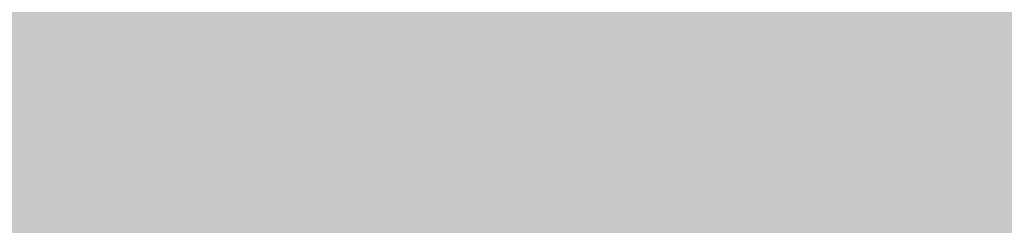
# Model space of a CAD drawing. Units: feet. Extents: x 3168 to 4724, y 827 to 1477.
# Tile 154 of 256: x 3301.19778 to 3301.26573, y 1099.00068 to 1099.01485. Entities that reach past the tile are written whole.
import ezdxf

# ---------------------------------------------------------------- set-up
doc = ezdxf.new("R2010")
doc.units = ezdxf.units.FT
doc.layers.add('A-ELEV', color=7, linetype='Continuous', lineweight=35)
doc.layers.add('A-ELEV-PATT', color=8, linetype='Continuous', lineweight=13)

msp = doc.modelspace()

# ---------------------------------------------------------------- hatches: boundary and pattern name
at = {"layer": 'A-ELEV-PATT'}
h = msp.add_hatch(color=256, dxfattribs=at)
h.dxf.hatch_style = 1
edge = h.paths.add_edge_path()
edge.add_ellipse((3552.905762, 979.220141), major_axis=(36.744924, 0), ratio=0.484848485, start_angle=0, end_angle=360)
edge = h.paths.add_edge_path()
edge.add_ellipse((3559.891637, 929.252282), major_axis=(36.744924, 0), ratio=0.484848485, start_angle=0, end_angle=360)
edge = h.paths.add_edge_path()
edge.add_line((3299.31681, 1198.606081), (3479.916714, 1198.606081))
edge.add_line((3479.916714, 1198.606081), (3479.916714, 1209.86857))
edge.add_spline(control_points=[(3479.916714, 1209.86857), (3464.301157, 1209.86857), (3448.685601, 1209.86857), (3410.949139, 1209.86857), (3388.828234, 1209.86857), (3355.646876, 1209.86857), (3344.586423, 1209.86857), (3327.995745, 1209.86857), (3322.465518, 1209.86857), (3314.170179, 1209.86857), (3311.405066, 1209.86857), (3307.257396, 1209.86857), (3305.874839, 1209.86857), (3303.801005, 1209.86857), (3303.109726, 1209.86857), (3302.072809, 1209.86857), (3301.72717, 1209.86857), (3301.208711, 1209.86857), (3301.035891, 1209.86857), (3300.776662, 1209.86857), (3300.690252, 1209.86857), (3300.560638, 1209.86857), (3300.517433, 1209.86857), (3300.452625, 1209.86857), (3300.431023, 1209.86857), (3300.398619, 1209.86857), (3300.387818, 1209.86857), (3300.366216, 1209.86857), (3300.345676, 1209.86857), (3300.345548, 1209.86857), (3300.345505, 1209.86857), (3300.343304, 1209.86857), (3300.341146, 1209.868571), (3300.337909, 1209.868571), (3300.33683, 1209.868572), (3300.333942, 1209.868573), (3300.332133, 1209.868574), (3300.325515, 1209.868577), (3300.320706, 1209.868581), (3300.310925, 1209.868592), (3300.305952, 1209.868598), (3300.290511, 1209.868623), (3300.280045, 1209.868646), (3300.232425, 1209.868777), (3300.195298, 1209.868954), (3299.951068, 1209.870608), (3299.744824, 1209.874326), (3299.436827, 1209.883257), (3299.334389, 1209.886792), (3299.181079, 1209.89292), (3299.130033, 1209.895099), (3298.652217, 1209.916801), (3298.22946, 1209.945718), (3297.601631, 1210.002367), (3297.393404, 1210.023464), (3297.082652, 1210.058309), (3296.979332, 1210.070458), (3296.292954, 1210.154861), (3295.718148, 1210.243356), (3294.868717, 1210.39885), (3294.5877, 1210.454478), (3294.169341, 1210.543349), (3294.030415, 1210.573878), (3291.707149, 1211.1012), (3289.65359, 1211.813435), (3285.776259, 1213.563988), (3283.95141, 1214.603478), (3280.512159, 1216.98008), (3278.897241, 1218.317592), (3276.379914, 1220.829489), (3275.416042, 1221.917738), (3274.039342, 1223.7077), (3273.581043, 1224.349535), (3273.143228, 1225.016316)], knot_values=[39.119033, 39.119033, 39.119033, 39.119033, 39.286353, 39.286353, 39.523379, 39.523379, 39.641892, 39.641892, 39.701148, 39.701148, 39.730777, 39.730777, 39.745591, 39.745591, 39.752998, 39.752998, 39.756701, 39.756701, 39.758553, 39.758553, 39.759479, 39.759479, 39.759942, 39.759942, 39.760173, 39.760173, 39.760289, 39.760289, 39.760405, 39.760405, 39.760463, 39.760463, 39.763389, 39.763389, 39.764851, 39.764851, 39.767304, 39.767304, 39.773825, 39.773825, 39.78057, 39.78057, 39.79477, 39.79477, 39.845194, 39.845194, 40.126715, 40.126715, 40.267476, 40.267476, 40.337856, 40.337856, 40.927023, 40.927023, 41.221606, 41.221606, 41.368898, 41.368898, 42.202622, 42.202622, 42.619485, 42.619485, 42.827916, 42.827916, 46.118323, 46.118323, 49.408731, 49.408731, 52.699139, 52.699139, 54.927489, 54.927489, 56.104228, 56.104228, 56.104228, 56.104228], weights=[1, 1, 1, 1, 1, 1, 1, 1, 1, 1, 1, 1, 1, 1, 1, 1, 1, 1, 1, 1, 1, 1, 1, 1, 1, 1, 1, 1, 1, 1, 1, 1, 1, 1, 1, 1, 1, 1, 1, 1, 1, 1, 1, 1, 1, 1, 1, 1, 1, 1, 1, 1, 1, 1, 1, 1, 1, 1, 1, 1, 1, 1, 1, 1, 1, 1, 1, 1, 1, 1, 1, 1, 1, 1], degree=3, periodic=0)
edge.add_line((3273.143228, 1225.016316), (3273.143228, 1099.016316))
edge.add_line((3273.143228, 1099.016316), (3299.31681, 1099.016316))
edge.add_line((3299.31681, 1099.016316), (3299.31681, 1198.606081))
edge = h.paths.add_edge_path()
edge.add_line((3304.758443, 1324.15806), (3479.916714, 1324.15806))
edge.add_line((3479.916714, 1324.15806), (3479.916714, 1335.714618))
edge.add_line((3479.916714, 1335.714618), (3269.161628, 1335.714618))
edge.add_spline(control_points=[(3269.161628, 1335.714618), (3264.024231, 1335.714618), (3258.364118, 1328.958189), (3259.264311, 1323.900274)], knot_values=[0, 0, 0, 0, 15.412191, 15.412191, 15.412191, 15.412191], degree=3, periodic=0)
edge.add_line((3259.264311, 1323.900274), (3265.516849, 1288.769135))
edge.add_line((3265.516849, 1288.769135), (3275.265103, 1261.545626))
edge.add_line((3275.265103, 1261.545626), (3304.758443, 1261.545626))
edge.add_line((3304.758443, 1261.545626), (3304.758443, 1324.15806))
h = msp.add_hatch(color=256, dxfattribs=at)
h.dxf.hatch_style = 1
h.paths.add_polyline_path([(3384.525247, 1099.016316), (3335.029168, 1099.016316), (3299.31681, 1099.016316), (3273.143228, 1099.016316), (3217.565364, 1099.016316), (3168.069285, 827.11626), (3335.029168, 827.11626)])

# ---------------------------------------------------------------- linework, layer by layer
at = {"layer": 'A-ELEV'}
msp.add_open_spline([(3808.5202, 1099.016316), (3808.5202, 1141.413235), (3808.5202, 1183.810154), (3808.5202, 1226.635324), (3808.5202, 1227.063576), (3808.5202, 1227.491828), (3811.491871, 1248.994673), (3814.463542, 1270.497518), (3817.46523, 1292.217564), (3817.495247, 1292.434764), (3817.525264, 1292.651964), (3817.572801, 1310.106748), (3817.620339, 1327.561532), (3817.667877, 1345.016316), (3817.667877, 1345.457962), (3817.667877, 1345.899608), (3817.667877, 1346.456047), (3817.667877, 1346.57084), (3817.667877, 1346.752887), (3817.667877, 1346.820142), (3817.667877, 1346.93487), (3817.667877, 1346.982345), (3817.667877, 1347.038587), (3817.667877, 1347.047356), (3817.667877, 1347.073661), (3817.667877, 1347.059303), (3817.667877, 1347.061545), (3817.667876, 1347.062667), (3817.667875, 1347.066031), (3817.667874, 1347.068274), (3817.66787, 1347.075001), (3817.667866, 1347.079486), (3817.667849, 1347.092937), (3817.667833, 1347.101902), (3817.667766, 1347.12879), (3817.667699, 1347.146705), (3817.667432, 1347.200421), (3817.667165, 1347.236192), (3817.6661, 1347.343385), (3817.665038, 1347.414686), (3817.660812, 1347.628095), (3817.656608, 1347.769708), (3817.63997, 1348.192487), (3817.623509, 1348.471586), (3817.559094, 1349.300067), (3817.496121, 1349.840588), (3817.255432, 1351.424156), (3817.026318, 1352.428785), (3816.306871, 1354.888914), (3815.743745, 1356.268727), (3814.463959, 1358.81921), (3813.746413, 1359.990968), (3812.195838, 1362.172343), (3811.362245, 1363.182124), (3809.588836, 1365.069009), (3808.648816, 1365.946105), (3806.654262, 1367.579616), (3805.599702, 1368.336154), (3803.352891, 1369.722327), (3802.160535, 1370.352386), (3799.600813, 1371.453586), (3798.232688, 1371.925481), (3795.280084, 1372.634624), (3793.693148, 1372.872068), (3791.869441, 1372.92648), (3791.740861, 1372.92922), (3791.353371, 1372.934101), (3791.092707, 1372.932901), (3790.304116, 1372.915068), (3789.769543, 1372.884195), (3789.20919, 1372.830236), (3789.190622, 1372.828424), (3789.134892, 1372.822912), (3789.097705, 1372.819137), (3789.048445, 1372.814008), (3789.0364, 1372.812743), (3789.000256, 1372.808918), (3788.976147, 1372.806325), (3788.949405, 1372.803404), (3788.946786, 1372.803118), (3788.942567, 1372.802655), (3788.940967, 1372.80248), (3788.938572, 1372.802217), (3788.937777, 1372.802129), (3788.935391, 1372.801867), (3788.867535, 1372.794402), (3788.756866, 1372.782228), (3788.701532, 1372.776141), (3788.53553, 1372.75788), (3788.424861, 1372.745707), (3788.092856, 1372.709185), (3787.871519, 1372.684837), (3787.207509, 1372.611793), (3786.764835, 1372.563097), (3785.436814, 1372.417009), (3784.551467, 1372.319617), (3781.895425, 1372.027442), (3780.12473, 1371.832658), (3774.812646, 1371.248307), (3771.271256, 1370.858739), (3760.647088, 1369.690037), (3753.56431, 1368.910902), (3732.315973, 1366.573498), (3718.150416, 1365.015228), (3694.006758, 1362.359326), (3684.028657, 1361.261694), (3674.050557, 1360.164062), (3664.600662, 1360.164062), (3655.150767, 1360.164062), (3626.801081, 1360.164062), (3607.901291, 1360.164062), (3551.20192, 1360.164062), (3513.40234, 1360.164062), (3467.725182, 1360.164062), (3459.847604, 1360.164062), (3436.214873, 1360.164062), (3420.459718, 1360.164062), (3373.194255, 1360.164062), (3341.683946, 1360.164062), (3302.848162, 1360.164062), (3295.522686, 1360.164062), (3286.038292, 1360.164062), (3283.879372, 1360.164062), (3277.402613, 1360.164062), (3273.084773, 1360.164062), (3267.732851, 1360.164062), (3266.698768, 1360.164062), (3263.59652, 1360.164062), (3261.528355, 1360.164062), (3259.236943, 1360.164062), (3259.013697, 1360.164062), (3258.343958, 1360.164062), (3257.897466, 1360.164062), (3257.430998, 1360.164062), (3257.411022, 1360.164062), (3257.370573, 1360.164062), (3257.37547, 1360.164062), (3257.374598, 1360.164062), (3257.373937, 1360.164062), (3257.371956, 1360.164062), (3257.370635, 1360.164061), (3257.366673, 1360.16406), (3257.364032, 1360.164059), (3257.356109, 1360.164053), (3257.350828, 1360.164047), (3257.334987, 1360.164023), (3257.32443, 1360.163998), (3257.292769, 1360.163899), (3257.271676, 1360.163799), (3257.208439, 1360.163398), (3257.166337, 1360.162995), (3257.040206, 1360.161388), (3256.956349, 1360.159783), (3256.705504, 1360.153393), (3256.53924, 1360.147036), (3256.04357, 1360.121916), (3255.717296, 1360.097102), (3254.752446, 1360.000481), (3254.127968, 1359.906513), (3252.180067, 1359.525332), (3250.941574, 1359.143991), (3248.670175, 1358.24329), (3247.635739, 1357.723834), (3245.732632, 1356.603471), (3244.863388, 1356.00206), (3243.253108, 1354.742865), (3242.511972, 1354.084731), (3240.751052, 1352.344781), (3239.800961, 1351.229574), (3238.087769, 1348.87244), (3237.324685, 1347.630355), (3235.98251, 1344.971632), (3235.402205, 1343.554907), (3234.591081, 1340.815458), (3234.310882, 1339.54355), (3233.97649, 1336.802561), (3233.922113, 1335.330877), (3234.148916, 1332.591269), (3234.349529, 1331.367201), (3234.719893, 1329.999367), (3234.752423, 1329.883362), (3234.853619, 1329.534797), (3234.925892, 1329.301685), (3235.024836, 1329.002552), (3235.046924, 1328.936928), (3235.077639, 1328.847239), (3235.085924, 1328.823198), (3235.110939, 1328.751064), (3235.127828, 1328.702962), (3235.147992, 1328.646242), (3235.151059, 1328.637632), (3235.156096, 1328.623526), (3235.158061, 1328.61803), (3235.160209, 1328.61203), (3235.165612, 1328.596943), (3235.180099, 1328.556486), (3235.190263, 1328.528101), (3235.220756, 1328.442946), (3235.241084, 1328.386176), (3235.302069, 1328.215865), (3235.342726, 1328.102325), (3235.464696, 1327.761704), (3235.54601, 1327.534623), (3235.78995, 1326.853381), (3235.952577, 1326.39922), (3236.440459, 1325.036736), (3236.765713, 1324.128414), (3237.741475, 1321.403446), (3238.391983, 1319.586801), (3240.343508, 1314.136866), (3241.644525, 1310.503576), (3245.547574, 1299.603706), (3248.149607, 1292.337126), (3255.955706, 1270.537385), (3261.159772, 1256.004225), (3267.387618, 1238.612001), (3268.411397, 1235.752937), (3269.510378, 1232.683864), (3269.585579, 1232.473854), (3269.706612, 1232.135851), (3269.752444, 1232.007857), (3269.827329, 1231.79873), (3269.856382, 1231.717595), (3269.906325, 1231.578122), (3269.927215, 1231.519782), (3269.972468, 1231.393406), (3269.996831, 1231.325368), (3270.026503, 1231.242506), (3270.031811, 1231.227681), (3270.040282, 1231.204024), (3270.039224, 1231.206979), (3270.039359, 1231.206601), (3270.039427, 1231.206412), (3270.03963, 1231.205846), (3270.039765, 1231.205468), (3270.040171, 1231.204335), (3270.040442, 1231.203579), (3270.041254, 1231.201313), (3270.041796, 1231.199802), (3270.04342, 1231.195269), (3270.044504, 1231.192248), (3270.047756, 1231.183185), (3270.049926, 1231.177145), (3270.056442, 1231.159028), (3270.060793, 1231.146957), (3270.073867, 1231.110761), (3270.082613, 1231.086656), (3270.108936, 1231.014413), (3270.1266, 1230.96635), (3270.179934, 1230.822457), (3270.215947, 1230.726923), (3270.325323, 1230.441508), (3270.400026, 1230.252811), (3270.629249, 1229.691444), (3270.788883, 1229.323501), (3271.286488, 1228.238319), (3271.6431, 1227.539755), (3272.775859, 1225.515277), (3273.614169, 1224.260502), (3275.416042, 1221.917738), (3276.379914, 1220.829489), (3278.897241, 1218.317592), (3280.512159, 1216.98008), (3283.95141, 1214.603478), (3285.776259, 1213.563988), (3289.65359, 1211.813435), (3291.707149, 1211.1012), (3294.030415, 1210.573878), (3294.169341, 1210.543349), (3294.5877, 1210.454478), (3294.868717, 1210.39885), (3295.718148, 1210.243356), (3296.292954, 1210.154861), (3296.979332, 1210.070458), (3297.082652, 1210.058309), (3297.393404, 1210.023464), (3297.601631, 1210.002367), (3298.22946, 1209.945718), (3298.652217, 1209.916801), (3299.130033, 1209.895099), (3299.181079, 1209.89292), (3299.334389, 1209.886792), (3299.436827, 1209.883257), (3299.744824, 1209.874326), (3299.951068, 1209.870608), (3300.195298, 1209.868954), (3300.232425, 1209.868777), (3300.280045, 1209.868646), (3300.290511, 1209.868623), (3300.305952, 1209.868598), (3300.310925, 1209.868592), (3300.320706, 1209.868581), (3300.325515, 1209.868577), (3300.332133, 1209.868574), (3300.333942, 1209.868573), (3300.33683, 1209.868572), (3300.337909, 1209.868571), (3300.341146, 1209.868571), (3300.343304, 1209.86857), (3300.345505, 1209.86857), (3300.345548, 1209.86857), (3300.345676, 1209.86857), (3300.366216, 1209.86857), (3300.387818, 1209.86857), (3300.398619, 1209.86857), (3300.431023, 1209.86857), (3300.452625, 1209.86857), (3300.517433, 1209.86857), (3300.560638, 1209.86857), (3300.690252, 1209.86857), (3300.776662, 1209.86857), (3301.035891, 1209.86857), (3301.208711, 1209.86857), (3301.72717, 1209.86857), (3302.072809, 1209.86857), (3303.109726, 1209.86857), (3303.801005, 1209.86857), (3305.874839, 1209.86857), (3307.257396, 1209.86857), (3311.405066, 1209.86857), (3314.170179, 1209.86857), (3322.465518, 1209.86857), (3327.995745, 1209.86857), (3344.586423, 1209.86857), (3355.646876, 1209.86857), (3388.828234, 1209.86857), (3410.949139, 1209.86857), (3477.311855, 1209.86857), (3521.553665, 1209.86857), (3566.836184, 1209.86857), (3567.876892, 1209.86857), (3570.999017, 1209.86857), (3573.080433, 1209.86857), (3575.781396, 1209.86857), (3576.400943, 1209.86857), (3577.295821, 1209.86857), (3577.571152, 1209.86857), (3578.397146, 1209.86857), (3578.947808, 1209.86857), (3579.756491, 1209.86857), (3580.014511, 1209.86857), (3580.342737, 1209.86857), (3580.326865, 1209.86857), (3580.32717, 1209.86857), (3580.327323, 1209.86857), (3580.327781, 1209.86857), (3580.328086, 1209.86857), (3580.329002, 1209.86857), (3580.329613, 1209.86857), (3580.331445, 1209.86857), (3580.332667, 1209.86857), (3580.336332, 1209.868569), (3580.338775, 1209.868567), (3580.346107, 1209.868563), (3580.350995, 1209.868558), (3580.365663, 1209.86854), (3580.375445, 1209.868522), (3580.404801, 1209.868449), (3580.424386, 1209.868376), (3580.483183, 1209.868085), (3580.522437, 1209.867793), (3580.640361, 1209.866624), (3580.719195, 1209.865454), (3580.956315, 1209.860766), (3581.115222, 1209.85607), (3581.594164, 1209.83723), (3581.916419, 1209.818331), (3582.889947, 1209.742428), (3583.547986, 1209.666169), (3585.531827, 1209.360617), (3586.867216, 1209.053886), (3589.471545, 1208.252472), (3590.740241, 1207.757852), (3591.995451, 1207.158802), (3592.057809, 1207.12874), (3592.244242, 1207.037954), (3592.367676, 1206.976632), (3592.73528, 1206.790359), (3592.976752, 1206.663101), (3593.244539, 1206.516441), (3593.274731, 1206.499825), (3593.365115, 1206.449839), (3593.425113, 1206.416333), (3593.604314, 1206.315285), (3593.722725, 1206.247211), (3593.857212, 1206.168398), (3593.874362, 1206.158319), (3593.925741, 1206.128041), (3593.959899, 1206.107798), (3594.062086, 1206.046899), (3594.129827, 1206.006074), (3594.208436, 1205.958171), (3594.219683, 1205.951304), (3594.253391, 1205.930686), (3594.275819, 1205.916917), (3594.342972, 1205.875536), (3594.387563, 1205.847853), (3594.433616, 1205.81905), (3594.435256, 1205.818024), (3594.440175, 1205.814946), (3594.443453, 1205.812894), (3594.447123, 1205.810594), (3594.447516, 1205.810348), (3594.448695, 1205.80961), (3594.449481, 1205.809117), (3594.450366, 1205.808562), (3594.450466, 1205.8085), (3594.4506, 1205.808415), (3594.467399, 1205.797887), (3594.493269, 1205.781674), (3594.506204, 1205.773568), (3594.545008, 1205.749248), (3594.570878, 1205.733035), (3594.648487, 1205.684396), (3594.700226, 1205.651969), (3594.855444, 1205.554691), (3594.958922, 1205.489839), (3595.269357, 1205.295282), (3595.476314, 1205.165577), (3596.097185, 1204.776463), (3596.511099, 1204.517054), (3597.752841, 1203.738826), (3598.580669, 1203.220007), (3601.064152, 1201.663551), (3602.719807, 1200.625914), (3607.686774, 1197.513002), (3610.998085, 1195.437727), (3620.932018, 1189.211903), (3627.55464, 1185.061354), (3647.422507, 1172.609707), (3660.667751, 1164.308608), (3700.403484, 1139.405313), (3726.893973, 1122.803116), (3757.205715, 1103.806052), (3761.02697, 1101.411184), (3764.848224, 1099.016316), (3745.328271, 1099.016316), (3725.808319, 1099.016316), (3706.288366, 1099.016316), (3706.288366, 1108.453237), (3706.288366, 1117.890158), (3706.288366, 1127.327079), (3710.750754, 1127.327079), (3715.213143, 1127.327079), (3719.675531, 1127.327079)], degree=3, knots=[0, 0, 0, 0, 0.982037, 0.982037, 0.991957, 0.991957, 0.991957, 1.966522, 1.966522, 1.976367, 1.976367, 1.976367, 2.976367, 2.976367, 2.976367, 3.00169, 3.00169, 3.008272, 3.008272, 3.012129, 3.012129, 3.014851, 3.014851, 3.015353, 3.015353, 3.016359, 3.016359, 3.017365, 3.017365, 3.019376, 3.019376, 3.023398, 3.023398, 3.031442, 3.031442, 3.047531, 3.047531, 3.079708, 3.079708, 3.144063, 3.144063, 3.272772, 3.272772, 3.53019, 3.53019, 4.045026, 4.045026, 5.074698, 5.074698, 6.700878, 6.700878, 8.327058, 8.327058, 9.953238, 9.953238, 11.579418, 11.579418, 13.205598, 13.205598, 14.831778, 14.831778, 16.457958, 16.457958, 18.084138, 18.084138, 18.206872, 18.206872, 18.45234, 18.45234, 18.943275, 18.943275, 18.960093, 18.960093, 18.993729, 18.993729, 19.00461, 19.00461, 19.026374, 19.026374, 19.028737, 19.028737, 19.03018, 19.03018, 19.030897, 19.030897, 19.032332, 19.032332, 19.033766, 19.033766, 19.036636, 19.036636, 19.042374, 19.042374, 19.053851, 19.053851, 19.076805, 19.076805, 19.122714, 19.122714, 19.21453, 19.21453, 19.398163, 19.398163, 19.765429, 19.765429, 20.024128, 20.024128, 20.024128, 20.092031, 20.092031, 20.227836, 20.227836, 20.499446, 20.499446, 20.556051, 20.556051, 20.66926, 20.66926, 20.895678, 20.895678, 20.948316, 20.948316, 20.963829, 20.963829, 20.994855, 20.994855, 21.002285, 21.002285, 21.017146, 21.017146, 21.01875, 21.01875, 21.021959, 21.021959, 21.022102, 21.022102, 21.022249, 21.022249, 21.022708, 21.022708, 21.023627, 21.023627, 21.025464, 21.025464, 21.029138, 21.029138, 21.036486, 21.036486, 21.051183, 21.051183, 21.080575, 21.080575, 21.139361, 21.139361, 21.256932, 21.256932, 21.492073, 21.492073, 21.962356, 21.962356, 23.01002, 23.01002, 24.057684, 24.057684, 25.105348, 25.105348, 26.153011, 26.153011, 27.776787, 27.776787, 29.400562, 29.400562, 31.024337, 31.024337, 32.278801, 32.278801, 33.533265, 33.533265, 34.467568, 34.467568, 34.553971, 34.553971, 34.726776, 34.726776, 34.775309, 34.775309, 34.793079, 34.793079, 34.82862, 34.82862, 34.834979, 34.834979, 34.839039, 34.839039, 34.839411, 34.839411, 34.840285, 34.840285, 34.842034, 34.842034, 34.845531, 34.845531, 34.852525, 34.852525, 34.866512, 34.866512, 34.894488, 34.894488, 34.950439, 34.950439, 35.062342, 35.062342, 35.286147, 35.286147, 35.733758, 35.733758, 35.821815, 35.821815, 35.828283, 35.828283, 35.832225, 35.832225, 35.834724, 35.834724, 35.836521, 35.836521, 35.838617, 35.838617, 35.839073, 35.839073, 35.839345, 35.839345, 35.839617, 35.839617, 35.840161, 35.840161, 35.841249, 35.841249, 35.843425, 35.843425, 35.847778, 35.847778, 35.856482, 35.856482, 35.873891, 35.873891, 35.908709, 35.908709, 35.978345, 35.978345, 36.117617, 36.117617, 36.396161, 36.396161, 36.953248, 36.953248, 38.067423, 38.067423, 40.295772, 40.295772, 42.524122, 42.524122, 45.81453, 45.81453, 49.104937, 49.104937, 52.395345, 52.395345, 52.603776, 52.603776, 53.020639, 53.020639, 53.854363, 53.854363, 54.001655, 54.001655, 54.296238, 54.296238, 54.885405, 54.885405, 54.955785, 54.955785, 55.096546, 55.096546, 55.378067, 55.378067, 55.42849, 55.42849, 55.442691, 55.442691, 55.449436, 55.449436, 55.455957, 55.455957, 55.458409, 55.458409, 55.459872, 55.459872, 55.462798, 55.462798, 55.462856, 55.462856, 55.462972, 55.462972, 55.463088, 55.463088, 55.463319, 55.463319, 55.463782, 55.463782, 55.464708, 55.464708, 55.46656, 55.46656, 55.470263, 55.470263, 55.47767, 55.47767, 55.492484, 55.492484, 55.522112, 55.522112, 55.581369, 55.581369, 55.699882, 55.699882, 55.936907, 55.936907, 56.410959, 56.410959, 56.42211, 56.42211, 56.444413, 56.444413, 56.451051, 56.451051, 56.454001, 56.454001, 56.459901, 56.459901, 56.462666, 56.462666, 56.463418, 56.463418, 56.464171, 56.464171, 56.465675, 56.465675, 56.468684, 56.468684, 56.474702, 56.474702, 56.486738, 56.486738, 56.51081, 56.51081, 56.558955, 56.558955, 56.655243, 56.655243, 56.847821, 56.847821, 57.232975, 57.232975, 58.003284, 58.003284, 59.543901, 59.543901, 62.625137, 62.625137, 68.787607, 68.787607, 74.950078, 74.950078, 75.27336, 75.27336, 75.919923, 75.919923, 77.213051, 77.213051, 77.377769, 77.377769, 77.707206, 77.707206, 78.366079, 78.366079, 78.462532, 78.462532, 78.655436, 78.655436, 79.041245, 79.041245, 79.105735, 79.105735, 79.234714, 79.234714, 79.492672, 79.492672, 79.502197, 79.502197, 79.521249, 79.521249, 79.523534, 79.523534, 79.528103, 79.528103, 79.528682, 79.528682, 79.528885, 79.528885, 79.529089, 79.529089, 79.529495, 79.529495, 79.530308, 79.530308, 79.531935, 79.531935, 79.535187, 79.535187, 79.541693, 79.541693, 79.554704, 79.554704, 79.580725, 79.580725, 79.632769, 79.632769, 79.736856, 79.736856, 79.94503, 79.94503, 80.361377, 80.361377, 80.421435, 80.421435, 80.421435, 81.421435, 81.421435, 81.421435, 82.421435, 82.421435, 82.421435, 83.421435, 83.421435, 83.421435, 83.421435], dxfattribs=at)

doc.saveas('drawing.dxf')
